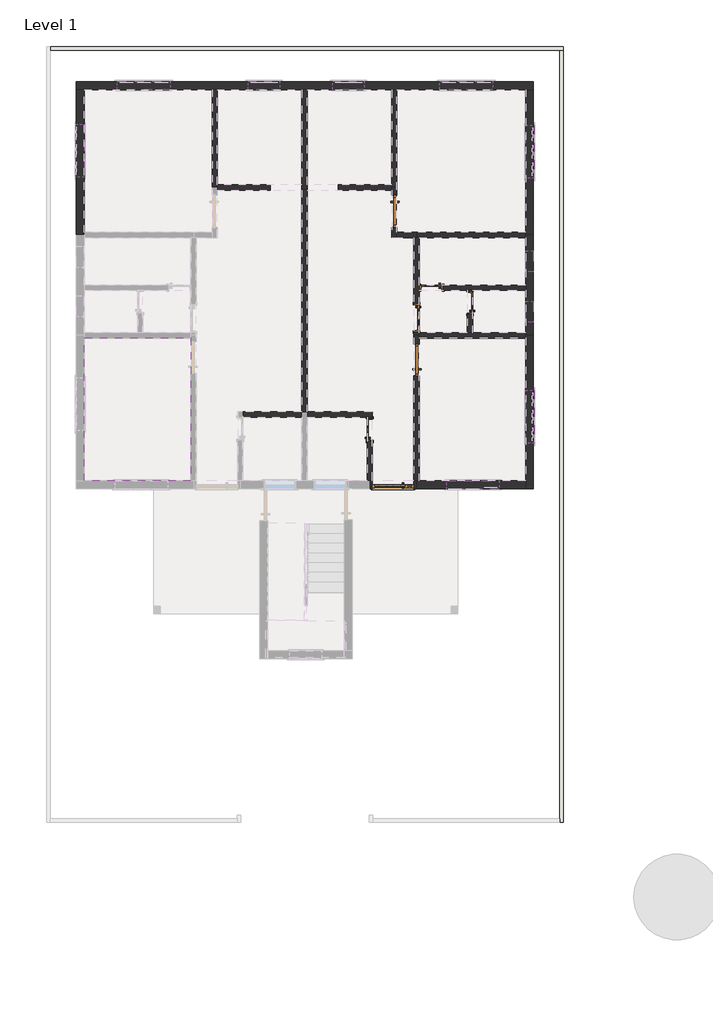
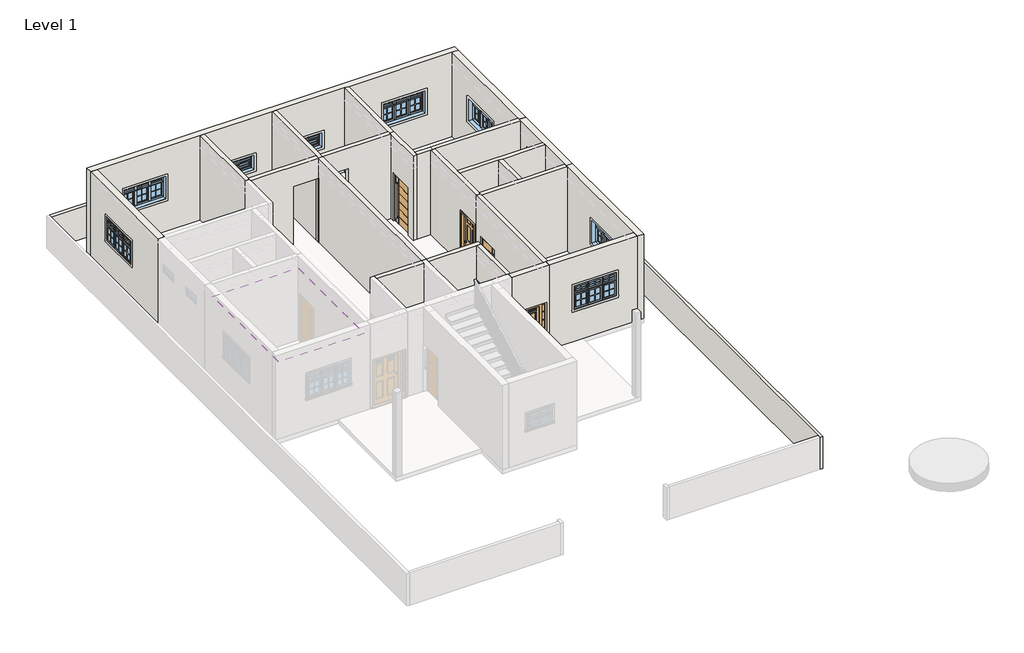
# One storey, part 2 of 4: 25 walls, 10 windows, 7 doors, 1 covering.
"""IFC4 building model written with IfcOpenShell, lengths in millimetres."""

from ifc_helpers import new_model, si_unit, frame, origin, place, context, project, spatial, polyline, outline, extrude, faceted_brep, transform, mapped, element, save
from components import door_3_ad1505b7, door_3_44036f4b, extsgl_w_side_panel_d749231e, m_door_interior_single_4_panel_wood_2_0346d007, m_door_interior_single_4_panel_wood_2_b7882c25, m_door_interior_single_6_panel_wood_750_x_2000mm_9b0189c3, fixed_2_8c8825d0, m_window_awning_double_vertical_3_7e34f04a, m_window_casement_triple_awning_triple_5_96d5a87e

model = new_model("IFC4")

# Units and contexts
model_context = context("Model", 3, world=origin())
ifc_project = project(units=[si_unit("LENGTHUNIT", "METRE", prefix="MILLI")], contexts=[model_context])

# Site, building, storey
site = spatial("IfcSite", under=ifc_project)
building = spatial("IfcBuilding", under=site)
storey = spatial("IfcBuildingStorey", under=building, Name="Level 1", Elevation=0.0)

# Covering
placement = place(None, origin())
element("IfcCovering", 1, ObjectType="2' x 4' ACT System", at=placement, inside=storey, context=model_context, shape_type="SweptSolid", body=[
    extrude(outline(polyline([(-10240.2299582, 8140.036641), (-13313.6299582, 8140.036641), (-13313.6299582, 12254.836641), (-10240.2299582, 12254.836641), (-10240.2299582, 8140.036641)])), frame((0.0, 0.0, 2743.2), z_axis=(0.0, 0.0, 1.0), x_axis=(1.0, 0.0, 0.0)), (0.0, 0.0, 1.0), 57.15),
])

# Doors
door_3_shape = door_3_ad1505b7(model_context)
element("IfcDoor", 2, ObjectType="3'", at=placement, inside=storey, context=model_context, shape_type="MappedRepresentation", body=[
    mapped(door_3_shape, transform((-4372.8299582, 15912.436641, 0.0), x_axis=(0.0, -1.0, 0.0), y_axis=(1.0, 0.0, 0.0), z_axis=(0.0, 0.0, 1.0))),
])
door_3_2_shape = door_3_44036f4b(model_context)
element("IfcDoor", 3, ObjectType="3'", at=placement, inside=storey, context=model_context, shape_type="MappedRepresentation", body=[
    mapped(door_3_2_shape, transform((-3737.8299582, 11619.836641, 0.0), x_axis=(0.0, 1.0, 0.0), y_axis=(-1.0, 0.0, 0.0), z_axis=(0.0, 0.0, 1.0))),
])
extsgl_w_side_panel_shape = extsgl_w_side_panel_d749231e(model_context)
element("IfcDoor", 4, ObjectType="ExtSgl w Side Panel", at=placement, inside=storey, context=model_context, shape_type="MappedRepresentation", body=[
    mapped(extsgl_w_side_panel_shape, transform((-4643.0299582, 8025.736641, 0.0), x_axis=(-1.0, 0.0, 0.0), y_axis=(0.0, -1.0, 0.0), z_axis=(0.0, 0.0, 1.0))),
])
m_door_interior_single_4_panel_wood_2_shape = m_door_interior_single_4_panel_wood_2_0346d007(model_context)
element("IfcDoor", 5, ObjectType="M_Door-Interior-Single-4_Panel-Wood : 2'", at=placement, inside=storey, context=model_context, shape_type="MappedRepresentation", body=[
    mapped(m_door_interior_single_4_panel_wood_2_shape, transform((-5087.2049582, 9613.236641, 0.0), x_axis=(0.0, 1.0, 0.0), y_axis=(-1.0, 0.0, 0.0), z_axis=(0.0, 0.0, 1.0))),
])
m_door_interior_single_4_panel_wood_2_2_shape = m_door_interior_single_4_panel_wood_2_b7882c25(model_context)
element("IfcDoor", 6, ObjectType="M_Door-Interior-Single-4_Panel-Wood : 2'", at=placement, inside=storey, context=model_context, shape_type="MappedRepresentation", body=[
    mapped(m_door_interior_single_4_panel_wood_2_2_shape, transform((-2185.2549582, 13270.836641, 0.0), x_axis=(0.0, 1.0, 0.0), y_axis=(-1.0, 0.0, 0.0), z_axis=(0.0, 0.0, 1.0))),
])
element("IfcDoor", 7, ObjectType="M_Door-Interior-Single-4_Panel-Wood : 2'", at=placement, inside=storey, context=model_context, shape_type="MappedRepresentation", body=[
    mapped(m_door_interior_single_4_panel_wood_2_2_shape, transform((-3306.0299582, 13705.811641, 0.0), x_axis=(-1.0, 0.0, 0.0), y_axis=(0.0, -1.0, 0.0), z_axis=(0.0, 0.0, 1.0))),
])
m_door_interior_single_6_panel_wood_750_x_2000mm_shape = m_door_interior_single_6_panel_wood_750_x_2000mm_9b0189c3(model_context)
element("IfcDoor", 8, ObjectType="M_Door-Interior-Single-6_Panel-Wood : 750 x 2000mm", at=placement, inside=storey, context=model_context, shape_type="MappedRepresentation", body=[
    mapped(m_door_interior_single_6_panel_wood_750_x_2000mm_shape, transform((-3734.6549582, 12839.036641, 0.0), x_axis=(0.0, -1.0, 0.0), y_axis=(1.0, 0.0, 0.0), z_axis=(0.0, 0.0, 1.0))),
])

# Walls
element("IfcWall", 9, ObjectType="Generic - 4\"", at=placement, inside=storey, context=model_context, shape_type="Brep", body=[
    faceted_brep([(-14304.2299582, 20560.636641, -152.4), (402.3700418, 20560.636641, -152.4), (503.9700418, 20560.636641, -152.4), (503.9700418, 20560.636641, 1066.8), (402.3700418, 20560.636641, 1066.8), (-14304.2299582, 20560.636641, 1066.8), (-14304.2299582, 20662.236641, -152.4), (-14304.2299582, 20662.236641, 1066.8), (503.9700418, 20662.236641, 1066.8), (503.9700418, 20662.236641, -152.4)], [[[0, 1, 2, 3, 4, 5]], [[6, 7, 8, 9]], [[2, 1, 0, 6, 9]], [[5, 4, 3, 8, 7]], [[0, 5, 7, 6]], [[3, 2, 9, 8]]]),
])
element("IfcWall", 10, ObjectType="Generic - 4\"", at=placement, inside=storey, context=model_context, shape_type="Brep", body=[
    faceted_brep([(402.3700418, 20560.636641, -152.4), (402.3700418, -1613.563359, -152.4), (402.3700418, -1715.163359, -152.4), (402.3700418, -1715.163359, 1066.8), (402.3700418, -1613.563359, 1066.8), (402.3700418, 20560.636641, 1066.8), (503.9700418, 20560.636641, -152.4), (503.9700418, 20560.636641, 1066.8), (503.9700418, -1715.163359, 1066.8), (503.9700418, -1715.163359, -152.4)], [[[0, 1, 2, 3, 4, 5]], [[6, 7, 8, 9]], [[2, 1, 0, 6, 9]], [[5, 4, 3, 8, 7]], [[0, 5, 7, 6]], [[3, 2, 9, 8]]]),
])
element("IfcWall", 11, ObjectType="Generic - 6\"", at=placement, inside=storey, context=model_context, shape_type="Brep", body=[
    faceted_brep([(-9630.6299582, 19417.636641, 0.0), (-9630.6299582, 16598.236641, 0.0), (-9630.6299582, 16598.236641, 3200.4), (-9630.6299582, 19417.636641, 3200.4), (-9478.2299582, 19417.636641, 0.0), (-9478.2299582, 19417.636641, 3200.4), (-9478.2299582, 16674.436641, 3200.4), (-9478.2299582, 16598.236641, 3200.4), (-9478.2299582, 16598.236641, 0.0), (-9478.2299582, 16674.436641, 0.0)], [[[0, 1, 2, 3]], [[4, 5, 6, 7, 8, 9]], [[1, 0, 4, 9, 8]], [[2, 1, 8, 7]], [[3, 2, 7, 6, 5]], [[0, 3, 5, 4]]]),
])
element("IfcWall", 12, ObjectType="Generic - 6\"", at=placement, inside=storey, context=model_context, shape_type="Brep", body=[
    faceted_brep([(-7039.8299582, 16522.036641, 0.0), (-7039.8299582, 16522.036641, 3200.4), (-9478.2299582, 16522.036641, 3200.4), (-9478.2299582, 16522.036641, 0.0), (-7956.9693204, 16522.036641, 0.0), (-7956.9693204, 16522.036641, 2438.4), (-7041.2238046, 16522.036641, 2438.4), (-7041.2238046, 16522.036641, 0.0), (-7039.8299582, 16674.436641, 3200.4), (-7039.8299582, 16674.436641, 0.0), (-7041.2238046, 16674.436641, 0.0), (-7041.2238046, 16674.436641, 2438.4), (-7956.9693204, 16674.436641, 2438.4), (-7956.9693204, 16674.436641, 0.0), (-9478.2299582, 16674.436641, 0.0), (-9478.2299582, 16674.436641, 3200.4), (-9478.2299582, 16598.236641, 0.0), (-7039.8299582, 16534.736641, 0.0), (-7039.8299582, 16534.736641, 3200.4), (-9478.2299582, 16598.236641, 3200.4)], [[[0, 1, 2, 3, 4, 5, 6, 7]], [[8, 9, 10, 11, 12, 13, 14, 15]], [[3, 16, 14, 13, 4]], [[9, 17, 0, 7, 10]], [[2, 1, 18, 8, 15, 19]], [[3, 2, 19, 15, 14, 16]], [[1, 0, 17, 9, 8, 18]], [[5, 12, 11, 6]], [[12, 5, 4, 13]], [[6, 11, 10, 7]]]),
])
element("IfcWall", 13, ObjectType="Generic - 6\"", at=placement, inside=storey, context=model_context, shape_type="Brep", body=[
    faceted_brep([(-7039.8299582, 19417.636641, 0.0), (-7039.8299582, 16674.436641, 0.0), (-7039.8299582, 16534.736641, 0.0), (-7039.8299582, 16534.736641, 3200.4), (-7039.8299582, 16674.436641, 3200.4), (-7039.8299582, 19417.636641, 3200.4), (-6887.4299582, 19417.636641, 0.0), (-6887.4299582, 19417.636641, 3200.4), (-6887.4299582, 16674.436641, 3200.4), (-6887.4299582, 16534.736641, 3200.4), (-6887.4299582, 16534.736641, 0.0), (-6887.4299582, 16674.436641, 0.0)], [[[0, 1, 2, 3, 4, 5]], [[6, 7, 8, 9, 10, 11]], [[2, 1, 0, 6, 11, 10]], [[3, 2, 10, 9]], [[5, 4, 3, 9, 8, 7]], [[0, 5, 7, 6]]]),
])
element("IfcWall", 14, ObjectType="Generic - 6\"", at=placement, inside=storey, context=model_context, shape_type="Brep", body=[
    faceted_brep([(-4449.0299582, 19417.636641, 0.0), (-4449.0299582, 16674.436641, 0.0), (-4449.0299582, 16598.236641, 0.0), (-4449.0299582, 16598.236641, 3200.4), (-4449.0299582, 16674.436641, 3200.4), (-4449.0299582, 19417.636641, 3200.4), (-4296.6299582, 19417.636641, 0.0), (-4296.6299582, 19417.636641, 3200.4), (-4296.6299582, 16598.236641, 3200.4), (-4296.6299582, 16598.236641, 0.0)], [[[0, 1, 2, 3, 4, 5]], [[6, 7, 8, 9]], [[2, 1, 0, 6, 9]], [[3, 2, 9, 8]], [[5, 4, 3, 8, 7]], [[0, 5, 7, 6]]]),
])
element("IfcWall", 15, ObjectType="Generic - 6\"", at=placement, inside=storey, context=model_context, shape_type="Brep", body=[
    faceted_brep([(-6887.4299582, 16674.436641, 0.0), (-6887.4299582, 16674.436641, 3200.4), (-4449.0299582, 16674.436641, 3200.4), (-4449.0299582, 16674.436641, 0.0), (-5985.1509554, 16674.436641, 0.0), (-5985.1509554, 16674.436641, 2438.4), (-6886.6436227, 16674.436641, 2438.4), (-6886.6436227, 16674.436641, 0.0), (-6887.4299582, 16522.036641, 3200.4), (-6887.4299582, 16522.036641, 0.0), (-6886.6436227, 16522.036641, 0.0), (-6886.6436227, 16522.036641, 2438.4), (-5985.1509554, 16522.036641, 2438.4), (-5985.1509554, 16522.036641, 0.0), (-4449.0299582, 16522.036641, 0.0), (-4449.0299582, 16522.036641, 3200.4), (-6887.4299582, 16534.736641, 0.0), (-4449.0299582, 16598.236641, 0.0), (-6887.4299582, 16534.736641, 3200.4), (-4449.0299582, 16598.236641, 3200.4)], [[[0, 1, 2, 3, 4, 5, 6, 7]], [[8, 9, 10, 11, 12, 13, 14, 15]], [[9, 16, 0, 7, 10]], [[3, 17, 14, 13, 4]], [[2, 1, 18, 8, 15, 19]], [[1, 0, 16, 9, 8, 18]], [[3, 2, 19, 15, 14, 17]], [[5, 12, 11, 6]], [[12, 5, 4, 13]], [[6, 11, 10, 7]]]),
])
element("IfcWall", 16, ObjectType="Generic - 6\"", at=placement, inside=storey, context=model_context, shape_type="Brep", body=[
    faceted_brep([(-4296.6299582, 15150.436641, 0.0), (-3814.0299582, 15150.436641, 0.0), (-3737.8299582, 15150.436641, 0.0), (-3737.8299582, 15150.436641, 3200.4), (-3814.0299582, 15150.436641, 3200.4), (-4296.6299582, 15150.436641, 3200.4), (-4296.6299582, 15302.836641, 0.0), (-4296.6299582, 15302.836641, 3200.4), (-3737.8299582, 15302.836641, 3200.4), (-3737.8299582, 15302.836641, 0.0)], [[[0, 1, 2, 3, 4, 5]], [[6, 7, 8, 9]], [[2, 1, 0, 6, 9]], [[3, 2, 9, 8]], [[5, 4, 3, 8, 7]], [[0, 5, 7, 6]]]),
])
element("IfcWall", 17, ObjectType="Generic - 6\"", at=placement, inside=storey, context=model_context, shape_type="Brep", body=[
    faceted_brep([(-3814.0299582, 12331.036641, 0.0), (-3814.0299582, 12331.036641, 3200.4), (-3814.0299582, 15150.436641, 3200.4), (-3814.0299582, 15150.436641, 0.0), (-3814.0299582, 13239.036641, 0.0), (-3814.0299582, 13239.036641, 2025.0), (-3814.0299582, 12439.036641, 2025.0), (-3814.0299582, 12439.036641, 0.0), (-3661.6299582, 12331.036641, 3200.4), (-3661.6299582, 12331.036641, 0.0), (-3661.6299582, 12407.236641, 0.0), (-3661.6299582, 12439.036641, 0.0), (-3661.6299582, 12439.036641, 2025.0), (-3661.6299582, 13239.036641, 2025.0), (-3661.6299582, 13239.036641, 0.0), (-3661.6299582, 13626.436641, 0.0), (-3661.6299582, 13778.836641, 0.0), (-3661.6299582, 15150.436641, 0.0), (-3661.6299582, 15150.436641, 3200.4), (-3661.6299582, 13778.836641, 3200.4), (-3661.6299582, 13626.436641, 3200.4), (-3661.6299582, 12407.236641, 3200.4), (-3737.8299582, 15150.436641, 0.0), (-3737.8299582, 15150.436641, 3200.4)], [[[0, 1, 2, 3, 4, 5, 6, 7]], [[8, 9, 10, 11, 12, 13, 14, 15, 16, 17, 18, 19, 20, 21]], [[3, 22, 17, 16, 15, 14, 4]], [[9, 0, 7, 11, 10]], [[1, 0, 9, 8]], [[2, 1, 8, 21, 20, 19, 18, 23]], [[3, 2, 23, 18, 17, 22]], [[6, 12, 11, 7]], [[12, 6, 5, 13]], [[13, 5, 4, 14]]]),
])
element("IfcWall", 18, ObjectType="Generic - 6\"", at=placement, inside=storey, context=model_context, shape_type="Brep", body=[
    faceted_brep([(-3661.6299582, 12254.836641, 0.0), (-588.2299582, 12254.836641, 0.0), (-588.2299582, 12254.836641, 3200.4), (-3661.6299582, 12254.836641, 3200.4), (-3661.6299582, 12407.236641, 0.0), (-3661.6299582, 12407.236641, 3200.4), (-2264.6299582, 12407.236641, 3200.4), (-2112.2299582, 12407.236641, 3200.4), (-588.2299582, 12407.236641, 3200.4), (-588.2299582, 12407.236641, 0.0), (-2112.2299582, 12407.236641, 0.0), (-2264.6299582, 12407.236641, 0.0), (-3661.6299582, 12331.036641, 0.0), (-588.2299582, 12331.036641, 0.0), (-588.2299582, 12331.036641, 3200.4), (-3661.6299582, 12331.036641, 3200.4)], [[[0, 1, 2, 3]], [[4, 5, 6, 7, 8, 9, 10, 11]], [[1, 0, 12, 4, 11, 10, 9, 13]], [[3, 2, 14, 8, 7, 6, 5, 15]], [[2, 1, 13, 9, 8, 14]], [[0, 3, 15, 5, 4, 12]]]),
])
element("IfcWall", 19, ObjectType="Generic - 6\"", at=placement, inside=storey, context=model_context, shape_type="SweptSolid", body=[
    extrude(outline(polyline([(12407.236641, 3200.4), (13626.436641, 3200.4), (13626.436641, 0.0), (13600.636641, 0.0), (13600.636641, 1853.8), (12941.036641, 1853.8), (12941.036641, 0.0), (12407.236641, 0.0), (12407.236641, 3200.4)])), frame((-2264.6299582, 0.0, 0.0), z_axis=(1.0, 0.0, 0.0), x_axis=(0.0, 1.0, 0.0)), (0.0, 0.0, 1.0), 152.4),
])
element("IfcWall", 20, ObjectType="Generic - 6\"", at=placement, inside=storey, context=model_context, shape_type="Brep", body=[
    faceted_brep([(-3661.6299582, 13778.836641, 3200.4), (-588.2299582, 13778.836641, 3200.4), (-588.2299582, 13778.836641, 0.0), (-2976.2299582, 13778.836641, 0.0), (-2976.2299582, 13778.836641, 1853.8), (-3635.8299582, 13778.836641, 1853.8), (-3635.8299582, 13778.836641, 0.0), (-3661.6299582, 13778.836641, 0.0), (-588.2299582, 13626.436641, 3200.4), (-2112.2299582, 13626.436641, 3200.4), (-2264.6299582, 13626.436641, 3200.4), (-3661.6299582, 13626.436641, 3200.4), (-3661.6299582, 13626.436641, 0.0), (-3635.8299582, 13626.436641, 0.0), (-3635.8299582, 13626.436641, 1853.8), (-2976.2299582, 13626.436641, 1853.8), (-2976.2299582, 13626.436641, 0.0), (-2264.6299582, 13626.436641, 0.0), (-2112.2299582, 13626.436641, 0.0), (-588.2299582, 13626.436641, 0.0)], [[[0, 1, 2, 3, 4, 5, 6, 7]], [[8, 9, 10, 11, 12, 13, 14, 15, 16, 17, 18, 19]], [[2, 19, 18, 17, 16, 3]], [[12, 7, 6, 13]], [[1, 0, 11, 10, 9, 8]], [[2, 1, 8, 19]], [[0, 7, 12, 11]], [[5, 14, 13, 6]], [[14, 5, 4, 15]], [[15, 4, 3, 16]]]),
])
element("IfcWall", 21, ObjectType="Generic - 6\"", at=placement, inside=storey, context=model_context, shape_type="Brep", body=[
    faceted_brep([(-8741.6299582, 9968.836641, 3200.4), (-8741.6299582, 9968.836641, 0.0), (-7039.8299582, 9968.836641, 0.0), (-7039.8299582, 9968.836641, 3200.4), (-8741.6299582, 10121.236641, 0.0), (-8741.6299582, 10121.236641, 3200.4), (-7039.8299582, 10121.236641, 3200.4), (-7039.8299582, 10121.236641, 0.0), (-7039.8299582, 10108.536641, 0.0), (-7039.8299582, 10108.536641, 3200.4)], [[[0, 1, 2, 3]], [[4, 5, 6, 7]], [[1, 4, 7, 8, 2]], [[5, 0, 3, 9, 6]], [[1, 0, 5, 4]], [[7, 6, 9, 3, 2, 8]]]),
    faceted_brep([(-5007.8299582, 9968.836641, 0.0), (-5007.8299582, 9968.836641, 3200.4), (-5160.2299582, 9968.836641, 3200.4), (-6887.4299582, 9968.836641, 3200.4), (-6887.4299582, 9968.836641, 0.0), (-5160.2299582, 9968.836641, 0.0), (-5007.8299582, 10121.236641, 3200.4), (-5007.8299582, 10121.236641, 0.0), (-6887.4299582, 10121.236641, 0.0), (-6887.4299582, 10121.236641, 3200.4), (-6887.4299582, 10108.536641, 0.0), (-6887.4299582, 10108.536641, 3200.4)], [[[0, 1, 2, 3, 4, 5]], [[6, 7, 8, 9]], [[7, 0, 5, 4, 10, 8]], [[1, 6, 9, 11, 3, 2]], [[1, 0, 7, 6]], [[9, 8, 10, 4, 3, 11]]]),
])
element("IfcWall", 22, ObjectType="Generic - 6\"", at=placement, inside=storey, context=model_context, shape_type="Brep", body=[
    faceted_brep([(-5160.2299582, 8140.036641, 3200.4), (-5160.2299582, 9968.836641, 3200.4), (-5160.2299582, 9968.836641, 0.0), (-5160.2299582, 9943.036641, 0.0), (-5160.2299582, 9943.036641, 1853.8), (-5160.2299582, 9283.436641, 1853.8), (-5160.2299582, 9283.436641, 0.0), (-5160.2299582, 8140.036641, 0.0), (-5007.8299582, 9968.836641, 3200.4), (-5007.8299582, 8140.036641, 3200.4), (-5007.8299582, 8140.036641, 1828.8), (-5007.8299582, 8140.036641, 0.0), (-5007.8299582, 9283.436641, 0.0), (-5007.8299582, 9283.436641, 1853.8), (-5007.8299582, 9943.036641, 1853.8), (-5007.8299582, 9943.036641, 0.0), (-5007.8299582, 9968.836641, 0.0), (-5084.0299582, 8140.036641, 0.0), (-5084.0299582, 8140.036641, 3200.4)], [[[0, 1, 2, 3, 4, 5, 6, 7]], [[8, 9, 10, 11, 12, 13, 14, 15, 16]], [[2, 16, 15, 3]], [[11, 17, 7, 6, 12]], [[1, 0, 18, 9, 8]], [[2, 1, 8, 16]], [[0, 7, 17, 11, 10, 9, 18]], [[14, 4, 3, 15]], [[4, 14, 13, 5]], [[5, 13, 12, 6]]]),
])
element("IfcWall", 23, ObjectType="Generic - 6\"", at=placement, inside=storey, context=model_context, shape_type="Brep", body=[
    faceted_brep([(-3814.0299582, 8140.036641, 3200.4), (-3814.0299582, 12331.036641, 3200.4), (-3814.0299582, 12331.036641, 0.0), (-3814.0299582, 12077.036641, 0.0), (-3814.0299582, 12077.036641, 1828.8), (-3814.0299582, 11162.636641, 1828.8), (-3814.0299582, 11162.636641, 0.0), (-3814.0299582, 8140.036641, 0.0), (-3661.6299582, 12331.036641, 3200.4), (-3661.6299582, 12254.836641, 3200.4), (-3661.6299582, 8140.036641, 3200.4), (-3661.6299582, 8140.036641, 0.0), (-3661.6299582, 11162.636641, 0.0), (-3661.6299582, 11162.636641, 1828.8), (-3661.6299582, 12077.036641, 1828.8), (-3661.6299582, 12077.036641, 0.0), (-3661.6299582, 12254.836641, 0.0), (-3661.6299582, 12331.036641, 0.0), (-3737.8299582, 8140.036641, 0.0), (-3758.6299582, 11162.636641, 0.0), (-3758.6299582, 11147.636641, 0.0), (-3681.6299582, 11147.636641, 0.0), (-3681.6299582, 11162.636641, 0.0), (-3681.6299582, 12077.036641, 0.0), (-3681.6299582, 12092.036641, 0.0), (-3758.6299582, 12092.036641, 0.0), (-3758.6299582, 12077.036641, 0.0), (-3737.8299582, 8140.036641, 3200.4), (-3681.6299582, 11162.636641, 1828.8), (-3681.6299582, 12077.036641, 1828.8), (-3758.6299582, 12077.036641, 1828.8), (-3758.6299582, 11162.636641, 1828.8), (-3681.6299582, 11147.636641, 1843.8), (-3758.6299582, 11147.636641, 1843.8), (-3758.6299582, 12092.036641, 1843.8), (-3681.6299582, 12092.036641, 1843.8)], [[[0, 1, 2, 3, 4, 5, 6, 7]], [[8, 9, 10, 11, 12, 13, 14, 15, 16, 17]], [[11, 18, 7, 6, 19, 20, 21, 22, 12]], [[2, 17, 16, 15, 23, 24, 25, 26, 3]], [[1, 0, 27, 10, 9, 8]], [[2, 1, 8, 17]], [[0, 7, 18, 11, 10, 27]], [[13, 28, 29, 14]], [[4, 30, 31, 5]], [[30, 4, 3, 26]], [[14, 29, 23, 15]], [[5, 31, 19, 6]], [[28, 13, 12, 22]], [[32, 33, 34, 35]], [[35, 34, 25, 24]], [[31, 30, 26, 25, 34, 33, 20, 19]], [[33, 32, 21, 20]], [[29, 28, 22, 21, 32, 35, 24, 23]]]),
])
element("IfcWall", 24, ObjectType="Generic - 6\"", at=placement, inside=storey, context=model_context, shape_type="Brep", body=[
    faceted_brep([(-7039.8299582, 16534.736641, 0.0), (-7039.8299582, 10121.236641, 0.0), (-7039.8299582, 10108.536641, 0.0), (-7039.8299582, 10108.536641, 3200.4), (-7039.8299582, 10121.236641, 3200.4), (-7039.8299582, 16534.736641, 3200.4), (-6887.4299582, 16534.736641, 0.0), (-6887.4299582, 16534.736641, 3200.4), (-6887.4299582, 10121.236641, 3200.4), (-6887.4299582, 10108.536641, 3200.4), (-6887.4299582, 10108.536641, 0.0), (-6887.4299582, 10121.236641, 0.0)], [[[0, 1, 2, 3, 4, 5]], [[6, 7, 8, 9, 10, 11]], [[2, 1, 0, 6, 11, 10]], [[3, 2, 10, 9]], [[5, 4, 3, 9, 8, 7]], [[0, 5, 7, 6]]]),
])
element("IfcWall", 25, ObjectType="Generic - 6\"", at=placement, inside=storey, context=model_context, shape_type="Brep", body=[
    faceted_brep([(-4449.0299582, 15150.436641, 3200.4), (-4449.0299582, 16522.036641, 3200.4), (-4449.0299582, 16598.236641, 3200.4), (-4449.0299582, 16598.236641, 0.0), (-4449.0299582, 16522.036641, 0.0), (-4449.0299582, 16369.636641, 0.0), (-4449.0299582, 16369.636641, 1828.8), (-4449.0299582, 15455.236641, 1828.8), (-4449.0299582, 15455.236641, 0.0), (-4449.0299582, 15150.436641, 0.0), (-4296.6299582, 16598.236641, 3200.4), (-4296.6299582, 15302.836641, 3200.4), (-4296.6299582, 15150.436641, 3200.4), (-4296.6299582, 15150.436641, 0.0), (-4296.6299582, 15302.836641, 0.0), (-4296.6299582, 15455.236641, 0.0), (-4296.6299582, 15455.236641, 1828.8), (-4296.6299582, 16369.636641, 1828.8), (-4296.6299582, 16369.636641, 0.0), (-4296.6299582, 16598.236641, 0.0), (-4393.6299582, 15455.236641, 0.0), (-4393.6299582, 15440.236641, 0.0), (-4316.6299582, 15440.236641, 0.0), (-4316.6299582, 15455.236641, 0.0), (-4316.6299582, 16369.636641, 0.0), (-4316.6299582, 16384.636641, 0.0), (-4393.6299582, 16384.636641, 0.0), (-4393.6299582, 16369.636641, 0.0), (-4393.6299582, 16369.636641, 1828.8), (-4393.6299582, 15455.236641, 1828.8), (-4316.6299582, 15455.236641, 1828.8), (-4316.6299582, 16369.636641, 1828.8), (-4316.6299582, 16384.636641, 1843.8), (-4316.6299582, 15440.236641, 1843.8), (-4393.6299582, 15440.236641, 1843.8), (-4393.6299582, 16384.636641, 1843.8)], [[[0, 1, 2, 3, 4, 5, 6, 7, 8, 9]], [[10, 11, 12, 13, 14, 15, 16, 17, 18, 19]], [[13, 9, 8, 20, 21, 22, 23, 15, 14]], [[3, 19, 18, 24, 25, 26, 27, 5, 4]], [[2, 1, 0, 12, 11, 10]], [[3, 2, 10, 19]], [[0, 9, 13, 12]], [[6, 28, 29, 7]], [[16, 30, 31, 17]], [[7, 29, 20, 8]], [[30, 16, 15, 23]], [[28, 6, 5, 27]], [[17, 31, 24, 18]], [[32, 33, 34, 35]], [[34, 33, 22, 21]], [[29, 28, 27, 26, 35, 34, 21, 20]], [[32, 35, 26, 25]], [[31, 30, 23, 22, 33, 32, 25, 24]]]),
])
element("IfcWall", 26, ObjectType="Generic - 6\"", at=placement, inside=storey, context=model_context, shape_type="Brep", body=[
    faceted_brep([(-3737.8299582, 15150.436641, 0.0), (-3661.6299582, 15150.436641, 0.0), (-588.2299582, 15150.436641, 0.0), (-588.2299582, 15150.436641, 3200.4), (-3661.6299582, 15150.436641, 3200.4), (-3737.8299582, 15150.436641, 3200.4), (-3737.8299582, 15302.836641, 0.0), (-3737.8299582, 15302.836641, 3200.4), (-588.2299582, 15302.836641, 3200.4), (-588.2299582, 15302.836641, 0.0), (-588.2299582, 15226.636641, 0.0), (-588.2299582, 15226.636641, 3200.4)], [[[0, 1, 2, 3, 4, 5]], [[6, 7, 8, 9]], [[2, 1, 0, 6, 9, 10]], [[5, 4, 3, 11, 8, 7]], [[0, 5, 7, 6]], [[3, 2, 10, 9, 8, 11]]]),
])
element("IfcWall", 27, ObjectType="Generic - 9\"", at=placement, inside=storey, context=model_context, shape_type="Brep", body=[
    faceted_brep([(-13542.2299582, 19417.636641, 0.0), (-13313.6299582, 19417.636641, 0.0), (-9630.6299582, 19417.636641, 0.0), (-9478.2299582, 19417.636641, 0.0), (-7039.8299582, 19417.636641, 0.0), (-6887.4299582, 19417.636641, 0.0), (-4449.0299582, 19417.636641, 0.0), (-4296.6299582, 19417.636641, 0.0), (-588.2299582, 19417.636641, 0.0), (-359.6299582, 19417.636641, 0.0), (-359.6299582, 19417.636641, 3200.4), (-588.2299582, 19417.636641, 3200.4), (-4296.6299582, 19417.636641, 3200.4), (-4449.0299582, 19417.636641, 3200.4), (-6887.4299582, 19417.636641, 3200.4), (-7039.8299582, 19417.636641, 3200.4), (-9478.2299582, 19417.636641, 3200.4), (-9630.6299582, 19417.636641, 3200.4), (-13313.6299582, 19417.636641, 3200.4), (-13542.2299582, 19417.636641, 3200.4), (-10837.1299582, 19417.636641, 2119.2), (-10837.1299582, 19417.636641, 1219.2), (-12361.1299582, 19417.636641, 1219.2), (-12361.1299582, 19417.636641, 2119.2), (-1540.7299582, 19417.636641, 2119.2), (-1540.7299582, 19417.636641, 1219.2), (-3064.7299582, 19417.636641, 1219.2), (-3064.7299582, 19417.636641, 2119.2), (-7674.8299582, 19417.636641, 1819.2), (-7674.8299582, 19417.636641, 1219.2), (-8589.2299582, 19417.636641, 1219.2), (-8589.2299582, 19417.636641, 1819.2), (-5236.4299582, 19417.636641, 1819.2), (-5236.4299582, 19417.636641, 1219.2), (-6150.8299582, 19417.636641, 1219.2), (-6150.8299582, 19417.636641, 1819.2), (-13542.2299582, 19646.236641, 0.0), (-13542.2299582, 19646.236641, 3200.4), (-359.6299582, 19646.236641, 3200.4), (-359.6299582, 19646.236641, 0.0), (-10837.1299582, 19646.236641, 2119.2), (-12361.1299582, 19646.236641, 2119.2), (-12361.1299582, 19646.236641, 1219.2), (-10837.1299582, 19646.236641, 1219.2), (-1540.7299582, 19646.236641, 2119.2), (-3064.7299582, 19646.236641, 2119.2), (-3064.7299582, 19646.236641, 1219.2), (-1540.7299582, 19646.236641, 1219.2), (-7674.8299582, 19646.236641, 1819.2), (-8589.2299582, 19646.236641, 1819.2), (-8589.2299582, 19646.236641, 1219.2), (-7674.8299582, 19646.236641, 1219.2), (-5236.4299582, 19646.236641, 1819.2), (-6150.8299582, 19646.236641, 1819.2), (-6150.8299582, 19646.236641, 1219.2), (-5236.4299582, 19646.236641, 1219.2)], [[[0, 1, 2, 3, 4, 5, 6, 7, 8, 9, 10, 11, 12, 13, 14, 15, 16, 17, 18, 19], [20, 21, 22, 23], [24, 25, 26, 27], [28, 29, 30, 31], [32, 33, 34, 35]], [[36, 37, 38, 39], [40, 41, 42, 43], [44, 45, 46, 47], [48, 49, 50, 51], [52, 53, 54, 55]], [[9, 8, 7, 6, 5, 4, 3, 2, 1, 0, 36, 39]], [[19, 18, 17, 16, 15, 14, 13, 12, 11, 10, 38, 37]], [[10, 9, 39, 38]], [[0, 19, 37, 36]], [[21, 20, 40, 43]], [[22, 21, 43, 42]], [[23, 22, 42, 41]], [[20, 23, 41, 40]], [[25, 24, 44, 47]], [[26, 25, 47, 46]], [[27, 26, 46, 45]], [[24, 27, 45, 44]], [[29, 28, 48, 51]], [[30, 29, 51, 50]], [[31, 30, 50, 49]], [[28, 31, 49, 48]], [[33, 32, 52, 55]], [[34, 33, 55, 54]], [[35, 34, 54, 53]], [[32, 35, 53, 52]]]),
])
element("IfcWall", 28, ObjectType="Generic - 9\"", at=placement, inside=storey, context=model_context, shape_type="Brep", body=[
    faceted_brep([(-588.2299582, 19417.636641, 0.0), (-588.2299582, 15302.836641, 0.0), (-588.2299582, 15226.636641, 0.0), (-588.2299582, 15226.636641, 3200.4), (-588.2299582, 15302.836641, 3200.4), (-588.2299582, 19417.636641, 3200.4), (-588.2299582, 16864.936641, 2119.2), (-588.2299582, 16864.936641, 1219.2), (-588.2299582, 18388.936641, 1219.2), (-588.2299582, 18388.936641, 2119.2), (-359.6299582, 19417.636641, 0.0), (-359.6299582, 19417.636641, 3200.4), (-359.6299582, 15226.636641, 3200.4), (-359.6299582, 15226.636641, 0.0), (-359.6299582, 16864.936641, 2119.2), (-359.6299582, 18388.936641, 2119.2), (-359.6299582, 18388.936641, 1219.2), (-359.6299582, 16864.936641, 1219.2)], [[[0, 1, 2, 3, 4, 5], [6, 7, 8, 9]], [[10, 11, 12, 13], [14, 15, 16, 17]], [[2, 1, 0, 10, 13]], [[3, 2, 13, 12]], [[5, 4, 3, 12, 11]], [[0, 5, 11, 10]], [[7, 6, 14, 17]], [[8, 7, 17, 16]], [[9, 8, 16, 15]], [[6, 9, 15, 14]]]),
])
element("IfcWall", 29, ObjectType="Generic - 9\"", at=placement, inside=storey, context=model_context, shape_type="Brep", body=[
    faceted_brep([(-588.2299582, 8140.036641, 0.0), (-3661.6299582, 8140.036641, 0.0), (-3737.8299582, 8140.036641, 0.0), (-3737.8299582, 8140.036641, 3200.4), (-3661.6299582, 8140.036641, 3200.4), (-588.2299582, 8140.036641, 3200.4), (-2867.8799582, 8140.036641, 2119.2), (-2867.8799582, 8140.036641, 1219.2), (-1343.8799582, 8140.036641, 1219.2), (-1343.8799582, 8140.036641, 2119.2), (-588.2299582, 7911.436641, 0.0), (-588.2299582, 7911.436641, 3200.4), (-3737.8299582, 7911.436641, 3200.4), (-3737.8299582, 7911.436641, 0.0), (-2867.8799582, 7911.436641, 2119.2), (-1343.8799582, 7911.436641, 2119.2), (-1343.8799582, 7911.436641, 1219.2), (-2867.8799582, 7911.436641, 1219.2)], [[[0, 1, 2, 3, 4, 5], [6, 7, 8, 9]], [[10, 11, 12, 13], [14, 15, 16, 17]], [[2, 1, 0, 10, 13]], [[3, 2, 13, 12]], [[5, 4, 3, 12, 11]], [[0, 5, 11, 10]], [[7, 6, 14, 17]], [[8, 7, 17, 16]], [[9, 8, 16, 15]], [[6, 9, 15, 14]]]),
])
element("IfcWall", 30, ObjectType="Generic - 9\"", at=placement, inside=storey, context=model_context, shape_type="Brep", body=[
    faceted_brep([(-588.2299582, 15226.636641, 0.0), (-588.2299582, 15150.436641, 0.0), (-588.2299582, 13778.836641, 0.0), (-588.2299582, 13626.436641, 0.0), (-588.2299582, 12407.236641, 0.0), (-588.2299582, 12331.036641, 0.0), (-588.2299582, 12331.036641, 3200.4), (-588.2299582, 12407.236641, 3200.4), (-588.2299582, 13626.436641, 3200.4), (-588.2299582, 13778.836641, 3200.4), (-588.2299582, 15150.436641, 3200.4), (-588.2299582, 15226.636641, 3200.4), (-588.2299582, 14159.836641, 2438.4), (-588.2299582, 14159.836641, 2133.6), (-588.2299582, 14769.436641, 2133.6), (-588.2299582, 14769.436641, 2438.4), (-588.2299582, 12712.036641, 2438.4), (-588.2299582, 12712.036641, 2133.6), (-588.2299582, 13321.636641, 2133.6), (-588.2299582, 13321.636641, 2438.4), (-359.6299582, 15226.636641, 0.0), (-359.6299582, 15226.636641, 3200.4), (-359.6299582, 12331.036641, 3200.4), (-359.6299582, 12331.036641, 0.0), (-359.6299582, 14159.836641, 2438.4), (-359.6299582, 14769.436641, 2438.4), (-359.6299582, 14769.436641, 2133.6), (-359.6299582, 14159.836641, 2133.6), (-359.6299582, 12712.036641, 2438.4), (-359.6299582, 13321.636641, 2438.4), (-359.6299582, 13321.636641, 2133.6), (-359.6299582, 12712.036641, 2133.6)], [[[0, 1, 2, 3, 4, 5, 6, 7, 8, 9, 10, 11], [12, 13, 14, 15], [16, 17, 18, 19]], [[20, 21, 22, 23], [24, 25, 26, 27], [28, 29, 30, 31]], [[5, 4, 3, 2, 1, 0, 20, 23]], [[6, 5, 23, 22]], [[11, 10, 9, 8, 7, 6, 22, 21]], [[0, 11, 21, 20]], [[12, 15, 25, 24]], [[15, 14, 26, 25]], [[14, 13, 27, 26]], [[13, 12, 24, 27]], [[16, 19, 29, 28]], [[19, 18, 30, 29]], [[18, 17, 31, 30]], [[17, 16, 28, 31]]]),
])
element("IfcWall", 31, ObjectType="Generic - 9\"", at=placement, inside=storey, context=model_context, shape_type="Brep", body=[
    faceted_brep([(-588.2299582, 12331.036641, 0.0), (-588.2299582, 12254.836641, 0.0), (-588.2299582, 8140.036641, 0.0), (-588.2299582, 7911.436641, 0.0), (-588.2299582, 7911.436641, 3200.4), (-588.2299582, 8140.036641, 3200.4), (-588.2299582, 12254.836641, 3200.4), (-588.2299582, 12331.036641, 3200.4), (-588.2299582, 9219.536641, 2119.2), (-588.2299582, 9219.536641, 1219.2), (-588.2299582, 10743.536641, 1219.2), (-588.2299582, 10743.536641, 2119.2), (-359.6299582, 12331.036641, 0.0), (-359.6299582, 12331.036641, 3200.4), (-359.6299582, 7911.436641, 3200.4), (-359.6299582, 7911.436641, 0.0), (-359.6299582, 9219.536641, 2119.2), (-359.6299582, 10743.536641, 2119.2), (-359.6299582, 10743.536641, 1219.2), (-359.6299582, 9219.536641, 1219.2)], [[[0, 1, 2, 3, 4, 5, 6, 7], [8, 9, 10, 11]], [[12, 13, 14, 15], [16, 17, 18, 19]], [[3, 2, 1, 0, 12, 15]], [[7, 6, 5, 4, 14, 13]], [[0, 7, 13, 12]], [[4, 3, 15, 14]], [[8, 11, 17, 16]], [[11, 10, 18, 17]], [[10, 9, 19, 18]], [[9, 8, 16, 19]]]),
])
element("IfcWall", 32, ObjectType="Generic - 9\"", at=placement, inside=storey, context=model_context, shape_type="Brep", body=[
    faceted_brep([(-5007.8299582, 8140.036641, 1828.8), (-5007.8299582, 8140.036641, 0.0), (-5084.0299582, 8140.036641, 0.0), (-5084.0299582, 8140.036641, 3200.4), (-5007.8299582, 8140.036641, 3200.4), (-3814.0299582, 8140.036641, 3200.4), (-3737.8299582, 8140.036641, 3200.4), (-3737.8299582, 8140.036641, 0.0), (-3814.0299582, 8140.036641, 0.0), (-3814.0299582, 8140.036641, 1828.8), (-5084.0299582, 7911.436641, 0.0), (-5007.8299582, 7911.436641, 0.0), (-5007.8299582, 7911.436641, 1828.8), (-3814.0299582, 7911.436641, 1828.8), (-3814.0299582, 7911.436641, 0.0), (-3737.8299582, 7911.436641, 0.0), (-3737.8299582, 7911.436641, 3200.4), (-5084.0299582, 7911.436641, 3200.4)], [[[0, 1, 2, 3, 4, 5, 6, 7, 8, 9]], [[10, 11, 12, 13, 14, 15, 16, 17]], [[8, 7, 15, 14]], [[2, 1, 11, 10]], [[3, 2, 10, 17]], [[6, 5, 4, 3, 17, 16]], [[7, 6, 16, 15]], [[13, 12, 0, 9]], [[12, 11, 1, 0]], [[14, 13, 9, 8]]]),
])
element("IfcWall", 33, ObjectType="Generic - 9\"", at=placement, inside=storey, context=model_context, shape_type="Brep", body=[
    faceted_brep([(-13313.6299582, 15226.636641, 0.0), (-13313.6299582, 15302.836641, 0.0), (-13313.6299582, 19417.636641, 0.0), (-13313.6299582, 19417.636641, 3200.4), (-13313.6299582, 15302.836641, 3200.4), (-13313.6299582, 15226.636641, 3200.4), (-13313.6299582, 18414.336641, 2119.2), (-13313.6299582, 18414.336641, 1219.2), (-13313.6299582, 16890.336641, 1219.2), (-13313.6299582, 16890.336641, 2119.2), (-13542.2299582, 15226.636641, 0.0), (-13542.2299582, 15226.636641, 3200.4), (-13542.2299582, 19417.636641, 3200.4), (-13542.2299582, 19417.636641, 0.0), (-13542.2299582, 18414.336641, 2119.2), (-13542.2299582, 16890.336641, 2119.2), (-13542.2299582, 16890.336641, 1219.2), (-13542.2299582, 18414.336641, 1219.2)], [[[0, 1, 2, 3, 4, 5], [6, 7, 8, 9]], [[10, 11, 12, 13], [14, 15, 16, 17]], [[2, 1, 0, 10, 13]], [[5, 4, 3, 12, 11]], [[0, 5, 11, 10]], [[3, 2, 13, 12]], [[6, 9, 15, 14]], [[9, 8, 16, 15]], [[8, 7, 17, 16]], [[7, 6, 14, 17]]]),
])

# Windows
fixed_2_shape = fixed_2_8c8825d0(model_context)
element("IfcWindow", 34, ObjectType="Fixed : 2'", at=placement, inside=storey, context=model_context, shape_type="MappedRepresentation", body=[
    mapped(fixed_2_shape, transform((-473.9299582, 14426.536641, 1219.2), x_axis=(0.0, -1.0, 0.0), y_axis=(1.0, 0.0, 0.0), z_axis=(0.0, 0.0, 1.0))),
])
element("IfcWindow", 35, ObjectType="Fixed : 2'", at=placement, inside=storey, context=model_context, shape_type="MappedRepresentation", body=[
    mapped(fixed_2_shape, transform((-473.9299582, 12978.736641, 1219.2), x_axis=(0.0, -1.0, 0.0), y_axis=(1.0, 0.0, 0.0), z_axis=(0.0, 0.0, 1.0))),
])
m_window_awning_double_vertical_3_shape = m_window_awning_double_vertical_3_7e34f04a(model_context)
element("IfcWindow", 36, ObjectType="M_Window-Awning-Double-Vertical : 4'", at=placement, inside=storey, context=model_context, shape_type="MappedRepresentation", body=[
    mapped(m_window_awning_double_vertical_3_shape, transform((-8132.0299582, 19531.936641, 319.2), x_axis=(1.0, 0.0, 0.0), y_axis=(0.0, 1.0, 0.0), z_axis=(0.0, 0.0, 1.0))),
])
element("IfcWindow", 37, ObjectType="M_Window-Awning-Double-Vertical : 4'", at=placement, inside=storey, context=model_context, shape_type="MappedRepresentation", body=[
    mapped(m_window_awning_double_vertical_3_shape, transform((-5693.6299582, 19531.936641, 319.2), x_axis=(1.0, 0.0, 0.0), y_axis=(0.0, 1.0, 0.0), z_axis=(0.0, 0.0, 1.0))),
])
m_window_casement_triple_awning_triple_5_shape = m_window_casement_triple_awning_triple_5_96d5a87e(model_context)
element("IfcWindow", 38, ObjectType="M_Window-Casement-Triple-Awning-Triple : 5'", at=placement, inside=storey, context=model_context, shape_type="MappedRepresentation", body=[
    mapped(m_window_casement_triple_awning_triple_5_shape, transform((-11599.1299582, 19531.936641, 319.2), x_axis=(1.0, 0.0, 0.0), y_axis=(0.0, 1.0, 0.0), z_axis=(0.0, 0.0, 1.0))),
])
element("IfcWindow", 39, ObjectType="M_Window-Casement-Triple-Awning-Triple : 5'", at=placement, inside=storey, context=model_context, shape_type="MappedRepresentation", body=[
    mapped(m_window_casement_triple_awning_triple_5_shape, transform((-13427.9299582, 17652.336641, 319.2), x_axis=(0.0, 1.0, 0.0), y_axis=(-1.0, 0.0, 0.0), z_axis=(0.0, 0.0, 1.0))),
])
element("IfcWindow", 40, ObjectType="M_Window-Casement-Triple-Awning-Triple : 5'", at=placement, inside=storey, context=model_context, shape_type="MappedRepresentation", body=[
    mapped(m_window_casement_triple_awning_triple_5_shape, transform((-2302.7299582, 19531.936641, 319.2), x_axis=(1.0, 0.0, 0.0), y_axis=(0.0, 1.0, 0.0), z_axis=(0.0, 0.0, 1.0))),
])
element("IfcWindow", 41, ObjectType="M_Window-Casement-Triple-Awning-Triple : 5'", at=placement, inside=storey, context=model_context, shape_type="MappedRepresentation", body=[
    mapped(m_window_casement_triple_awning_triple_5_shape, transform((-473.9299582, 17626.936641, 319.2), x_axis=(0.0, -1.0, 0.0), y_axis=(1.0, 0.0, 0.0), z_axis=(0.0, 0.0, 1.0))),
])
element("IfcWindow", 42, ObjectType="M_Window-Casement-Triple-Awning-Triple : 5'", at=placement, inside=storey, context=model_context, shape_type="MappedRepresentation", body=[
    mapped(m_window_casement_triple_awning_triple_5_shape, transform((-473.9299582, 9981.536641, 319.2), x_axis=(0.0, -1.0, 0.0), y_axis=(1.0, 0.0, 0.0), z_axis=(0.0, 0.0, 1.0))),
])
element("IfcWindow", 43, ObjectType="M_Window-Casement-Triple-Awning-Triple : 5'", at=placement, inside=storey, context=model_context, shape_type="MappedRepresentation", body=[
    mapped(m_window_casement_triple_awning_triple_5_shape, transform((-2105.8799582, 8025.736641, 319.2), x_axis=(-1.0, 0.0, 0.0), y_axis=(0.0, -1.0, 0.0), z_axis=(0.0, 0.0, 1.0))),
])

save(model, "model.ifc")

# Revit data of these elements
# Type "2' x 4' ACT System"
#   Assembly Code = "C3030210"
#   built-in parameter 1002203 = 1 (stored number, unit not read)
#   built-in parameter 1002202 = 1 (stored number, unit not read)
#   Layers, outside or top first: 0' - 1 5/8" "Default" (function 1); 0' - 0 5/8" "Acoustic Ceiling Tile 24 x 48" (function 5)
# Type "3'"
#   Type Mark = "9"
#   Water resistance = "up to Class E900, EN 12208:2001"
#   Uniclass2015Version = "v1.21"
#   Uniclass2015Reference = "Ss_25_30_20_30"
#   Uniclass2015Description = "Frame and door leaf system"
#   URL = "www.aluprof.com"
#   Type IFC Predefined Type = "USERDEFINED"
#   Right-hand / Left-hand door [instance default] = ""
#   Resistance to wind load = "up to Class C5/B5, EN 12210:2001"
#   Insert type = "ST"
#   Hardware [instance default] = ""
#   Product page = "https://aluprof.com/en/architects/offer/window-and-door-systems/panel-doors#visualisation"
#   Operation = "SinglePanelOutwardOpening"
#   Opening type = "Outward"
#   NBSReference = "25-50-20/125"
#   NBSDescription = "Frame and door leaf system"
#   Important = "The actual acceptable construction dimensions are dependent on the selection of profiles and hardware, glazing type, construction weight and the construction’s operating conditions. These should be determined by a suitably qualified person, and using ALUPROF’s calculation software"
#   IfcExportType = "USERDEFINED"
#   IfcExportAs = "IfcDoorType"
#   Handle type [instance default] = ""
#   Manufacturer = "ALUPROF SA"
#   Export Type to IFC As = "IfcDoorType"
#   Door sill type [instance default] = ""
#   Description = "External single-leaf panel door outward opening"
#   Model = "MB-86 ST Panel Door AD07"
#   Content of the recyclate in the material = "69.2%"
#   COBie.Type.WarrantyDurationParts = ""
#   COBie.Type.Name = ""
#   COBie.Type.Manufacturer = "ALUPROF SA"
#   COBie.Space.Name = ""
#   COBie.Floor.Name = ""
#   COBie.Facility.Name = ""
#   COBie.CreatedOn = ""
#   COBie.Component.WarrantyStartDate = ""
#   COBie.Component.Name = "MB-86 ST Panel Door AD07"
#   Burglar resistance = "RC2"
#   Air permeability = "up to Class 4, EN 12207:2001"
#   Width of the active leaf = 2' - 8.17717"
#   Placement in wall = 0' - 0.7874"
#   Thickness = 0' - 3.0315"
#   Height of the opening sash = 5' - 9.44094"
#   Handle Offset = 3' - 5.33858"
#   Rough Height = 6' - 2.40945"
#   Rough Width = 3' - 1.1811"
#   Height = 6' - 0"
#   Width = 3' - 0"
#   Construction depth = 0' - 3.0315"
#   Clear opening width = 2' - 3.94882"
#   Clear opening height = 5' - 8.47638"
#   Height of the array = 0' - 11.08136"
#   Schedule No. [instance default] = 1
#   Handrail [instance default] = yes
#   IsExternal = yes
#   Handle [instance default] = no
#   Door closer [instance default] = no
#   Function = 1
#   COBie.Type = yes
#   COBie = yes
#   Access control [instance default] = no
#   Panel = element 380416
#   Wall Closure = (empty or 0)
# Type "ExtSgl w Side Panel"
#   Type Mark = "14"
#   Operation = "SingleSwingRight"
#   Keynote = "L20"
#   Wrap Layers (Int) from Ext = 0' - 6.98819"
#   Wrap Layers (Ext) from Ext = 0' - 4.03543"
#   Thickness = 0' - 1.73228"
#   Stile Top of Lock rail = 3' - 3.37008"
#   Stile Top of Frieze Rail = 5' - 3.97638"
#   Stile Top Rail = 0' - 5.90551"
#   Stile Shutting = 0' - 4.92126"
#   Panelling Widths = 0' - 9.84252"
#   Stile Lock Rail = 0' - 6.88976"
#   Stile Intermediate/Frieze = 0' - 4.92126"
#   Stile Hanging = 0' - 4.92126"
#   Stile Bottom Rail = 0' - 6.88976"
#   Rough Width = 3' - 11"
#   Rough Height = 6' - 0"
#   O/A Frame Width = 0' - 2.51969"
#   Handle Z Distance = 3' - 3.37008"
#   Glazing Thickness = 0' - 0.94488"
#   Glazing Bar Thickness = 0' - 0.98425"
#   FrameWidth = 0' - 1.65354"
#   FrameOffset - External = 0' - 0.98425"
#   FrameDepth = 0' - 3.50394"
#   Door Panel Width = 2' - 11.70866"
#   Door Panel Thickness = 0' - 1.73228"
#   Door Panel Height = 5' - 7.66929"
#   Cill Thickness = 0' - 2.14567"
#   Cill Projection = 0' - 1.1811"
#   Handle X Distance = 0' - 2.95276"
#   Height = 6' - 0"
#   Structural Tolerance = 0' - 0.25591"
#   Tolerance = 0' - 0.11811"
#   Undercut = 0' - 0.15748"
#   Width = 3' - 11"
#   Cill Extension = 0' - 0.98425"
#   Cavity Closer Width = 0' - 1.9685"
#   Cavity Closer Offset from Ext = 0' - 4.03543"
#   Cavity Closer Depth = 0' - 3.34646"
#   Vis - SideLight Glazing Bars = yes
#   Vis - Ironmongery = yes
#   Vis - Cavity Closers = yes
#   Function = 1
#   Material Glass = Door - Glazing
#   Handle Style = element 390192
#   Material Door = Door - Panel
#   Material Ironmongery = Door - Handle
#   Wall Closure = (empty or 0)
# Type "M_Door-Interior-Single-4_Panel-Wood : 2'"
#   Type Mark = "13"
#   Assembly Code = "C1020300"
#   Analytic Construction = "Wooden"
#   Top Rail = 0' - 4.72441"
#   Thickness = 0' - 1.37795"
#   Thermal Resistance (R) = 2.5876 (h·ft²·°F)/BTU
#   Swing Angle [instance default] = 90.00°
#   Stiles = 0' - 4.72441"
#   Rough Width = 2' - 1.9685"
#   Rough Height = 6' - 0.98425"
#   Mullion = 0' - 4.52756"
#   Lock Rail = 0' - 7.87402"
#   Height = 6' - 0"
#   Width = 2' - 0"
#   Heat Transfer Coefficient (U) = 0.3865 BTU/(h·ft²·°F)
#   Bottom Rail = 0' - 9.05512"
#   Trim Material = Cherry
#   Panel Material = Cherry
#   Frame Material = Cherry
#   Door Handle Material = Aluminum
#   Visual Light Transmittance = 0
#   Solar Heat Gain Coefficient = 0
#   Wall Closure = (empty or 0)
#   Function = (empty or 0)
# Type "M_Door-Interior-Single-6_Panel-Wood : 750 x 2000mm"
#   Type Mark = "10"
#   Assembly Code = "C1020300"
#   Analytic Construction = "Wooden"
#   Top Rail = 0' - 4.72441"
#   Top Panel = 0' - 7.77559"
#   Thickness = 0' - 1.37795"
#   Thermal Resistance (R) = 2.5876 (h·ft²·°F)/BTU
#   Swing Angle [instance default] = 90.00°
#   Stiles = 0' - 4.72441"
#   Rough Width = 2' - 7.49606"
#   Rough Height = 6' - 7.72441"
#   Mullion = 0' - 4.52756"
#   Lock Rail = 0' - 7.87402"
#   Intermediate Rail = 0' - 4.52756"
#   Height = 6' - 6.74016"
#   Width = 2' - 5.52756"
#   Heat Transfer Coefficient (U) = 0.3865 BTU/(h·ft²·°F)
#   Bottom Rail = 0' - 9.05512"
#   Trim Material = Cherry
#   Panel Material = Cherry
#   Frame Material = Cherry
#   Door Handle Material = Aluminum
#   Visual Light Transmittance = 0
#   Solar Heat Gain Coefficient = 0
#   Wall Closure = (empty or 0)
#   Function = (empty or 0)
# Type "Generic - 4\""
#   Assembly Code = "B2010"
#   Layers, outside or top first: 0' - 4" no material (function 1)
# Type "Generic - 6\""
#   Assembly Code = "B2010"
#   Layers, outside or top first: 0' - 6" no material (function 1)
# Type "Generic - 9\""
#   Assembly Code = "B2010"
#   Layers, outside or top first: 0' - 9" no material (function 1)
# Type "Fixed : 2'"
#   Type Mark = "23"
#   Construction Type Id = "GSP4R"
#   Assembly Code = "B2020100"
#   Analytic Construction = "1/8 in Pilkington single glazing"
#   Visual Light Transmittance = 0.9
#   Solar Heat Gain Coefficient = 0.78
#   Heat Transfer Coefficient (U) = 0.6496 BTU/(h·ft²·°F)
#   Height = 1' - 0"
#   Default Sill Height = 3' - 0"
#   Width = 2' - 0"
#   Window Inset = 0' - 0 3/4"
#   Define Thermal Properties by = 1
#   Glass Pane Material = Glass
#   Sash Material = Sash
#   Wall Closure = (empty or 0)
# Type "M_Window-Awning-Double-Vertical : 4'"
#   Type Mark = "21"
#   Fire Rating = "0.5h"
#   Assembly Code = "B2020100"
#   Analytic Construction = "Double glazing - domestic"
#   Window Inset [instance default] = 0' - 0"
#   Wall Thickness [instance default] = 0' - 5.90551"
#   Visual Light Transmittance = 0.81
#   Top Sash Height Ratio = 0.5
#   Top Sash Height = 0' - 11.81102"
#   Thermal Resistance (R) = 1.8146 (h·ft²·°F)/BTU
#   Solar Heat Gain Coefficient = 0.76
#   Rough Width = 3' - 0.59055"
#   Rough Height = 2' - 0.2126"
#   Interior Wall Closure [instance default] = 0' - 2.15551"
#   Height = 1' - 11.62205"
#   Heat Transfer Coefficient (U) = 0.5511 BTU/(h·ft²·°F)
#   Frame Extension [instance default] = 0' - 0 1/4"
#   Exterior Wall Closure [instance default] = 0' - 1 1/4"
#   Extension Jamb [instance default] = 0' - 2.15551"
#   Default Sill Height = 2' - 11.43307"
#   Width = 3' - 0"
#   Top Muntin Visibility = yes
#   Interior Trim Visibility [instance default] = yes
#   Exterior Trim Visibility [instance default] = yes
#   Extension Jamb Visibility [instance default] = yes
#   Bottom Muntin Visibility = yes
#   Muntin Pattern = M_Muntin Pattern_2x2 : M_Muntin Pattern_2x2
#   Interior Trim Material = Wood - Stained
#   Interior Trim = M_Trim-Window-Interior-Flat : Picture Frame
#   Interior Frame Material = Wood - Stained
#   Glass Panel Material = Glass
#   Exterior Trim Material = Clad - White
#   Exterior Trim = M_Trim-Window-Exterior-Flat : with Sill
#   Exterior Frame Material = Clad - White
#   Wall Closure = (empty or 0)
# Type "M_Window-Casement-Triple-Awning-Triple : 5'"
#   Type Mark = "19"
#   Fire Rating = "0.5h"
#   Assembly Code = "B2020100"
#   Analytic Construction = "Double glazing - domestic"
#   Window Inset [instance default] = 0' - 0"
#   Wall Thickness [instance default] = 0' - 5.90551"
#   One Third Width = 1' - 8"
#   Visual Light Transmittance = 0.81
#   Transom Height = 0' - 11.81102"
#   Thermal Resistance (R) = 1.8146 (h·ft²·°F)/BTU
#   Solar Heat Gain Coefficient = 0.76
#   Sash Width = 1' - 7.16667"
#   Rough Width = 5' - 0.59055"
#   Rough Height = 3' - 0.02362"
#   Open Window Height = 1' - 11.62205"
#   Frame Extension [instance default] = 0' - 0 1/4"
#   Interior Wall Closure [instance default] = 0' - 2.15551"
#   Height = 2' - 11.43307"
#   Heat Transfer Coefficient (U) = 0.5511 BTU/(h·ft²·°F)
#   Exterior Wall Closure [instance default] = 0' - 1 1/4"
#   Extension Jamb [instance default] = 0' - 2.15551"
#   Default Sill Height = 2' - 11.43307"
#   Width = 5' - 0"
#   Top Side Muntin Visibility = yes
#   Top Middle Muntin Visibility = yes
#   Bottom Side Muntin Visibility = yes
#   Bottom Middle Muntin Visibility = yes
#   Interior Trim Visibility [instance default] = yes
#   Exterior Trim Visibility [instance default] = yes
#   Extension Jamb Visibility [instance default] = yes
#   Muntin Pattern = M_Muntin Pattern_2x2 : M_Muntin Pattern_2x2
#   Interior Trim Material = Wood - Stained
#   Interior Trim = M_Trim-Window-Interior-Flat : Picture Frame
#   Interior Frame Material = Wood - Stained
#   Glass Panel Material = Glass
#   Exterior Trim Material = Clad - White
#   Exterior Trim = M_Trim-Window-Exterior-Flat : with Sill
#   Exterior Frame Material = Clad - White
#   Wall Closure = (empty or 0)
# Element 1 (IfcCovering, "2' x 4' ACT System")
#   Height Offset From Level = 9' - 0"
#   Phase Created = New Construction
#   Materials on its faces: "Acoustic Ceiling Tile 24 x 48", "Default"
# Elements 2, 3 (IfcDoor, "3'")
#   Right-hand / Left-hand door = ""
#   Hardware = ""
#   Handle type = ""
#   Door sill type = ""
#   Schedule No. = 1
#   Handrail = yes
#   Handle = no
#   Door closer = no
#   Access control = no
#   Phase Created = New Construction
# Element 4 (IfcDoor, "ExtSgl w Side Panel")
#   Phase Created = New Construction
#   Materials on its faces: "Door - Panel", "Door - Handle", "Door - Glazing"
# Elements 5, 6, 7 (IfcDoor, "M_Door-Interior-Single-4_Panel-Wood : 2'")
#   Swing Angle = 90.00°
#   Phase Created = New Construction
#   Materials on its faces: "Cherry", "Aluminum"
# Element 8 (IfcDoor, "M_Door-Interior-Single-6_Panel-Wood : 750 x 2000mm")
#   Swing Angle = 90.00°
#   Phase Created = New Construction
#   Materials on its faces: "Cherry", "Aluminum"
# Elements 9, 10 (IfcWall, "Generic - 4\"")
#   built-in parameter 1001111 = -0' - 6"
#   Top Offset = 0' - 0"
#   Base Offset = -0' - 6"
#   Unconnected Height = 4' - 0"
#   wall height = 4' - 0"
#   Phase Created = New Construction
#   Base Constraint = Level 1
#   Materials on its faces: "LVW1", "Default Wall"
# Elements 11, 23 (IfcWall, "Generic - 6\"")
#   Top Offset = 0' - 0"
#   Base Offset = 0' - 0"
#   Unconnected Height = 10' - 6"
#   wall height = 10' - 6"
#   Phase Created = New Construction
#   Base Constraint = Level 1
#   Materials on its faces: "Default Wall", "BED ROOM WALL 1"
# Elements 12, 14, 16, 25 (IfcWall, "Generic - 6\"")
#   Top Offset = 0' - 0"
#   Base Offset = 0' - 0"
#   Unconnected Height = 10' - 6"
#   wall height = 10' - 6"
#   Phase Created = New Construction
#   Base Constraint = Level 1
#   Materials on its faces: "Default Wall", "BED ROOM WALL 2"
# Elements 13, 15 (IfcWall, "Generic - 6\"")
#   Top Offset = 0' - 0"
#   Base Offset = 0' - 0"
#   Unconnected Height = 10' - 6"
#   wall height = 10' - 6"
#   Phase Created = New Construction
#   Base Constraint = Level 1
#   Materials on its faces: "Default Wall", "BED ROOM WALL 2", "BED ROOM WALL 1"
# Elements 17, 19, 20, 21, 22 (IfcWall, "Generic - 6\"")
#   Top Offset = 0' - 0"
#   Base Offset = 0' - 0"
#   Unconnected Height = 10' - 6"
#   wall height = 10' - 6"
#   Phase Created = New Construction
#   Base Constraint = Level 1
#   Materials on its faces: "Default Wall", "BAW1"
# Element 18 (IfcWall, "Generic - 6\"")
#   Top Offset = 0' - 0"
#   Base Offset = 0' - 0"
#   Unconnected Height = 10' - 6"
#   wall height = 10' - 6"
#   Phase Created = New Construction
#   Base Constraint = Level 1
#   Materials on its faces: "Default Wall", "BED ROOM WALL 2", "BAW1"
# Element 24 (IfcWall, "Generic - 6\"")
#   Top Offset = 0' - 0"
#   Base Offset = 0' - 0"
#   Unconnected Height = 10' - 6"
#   wall height = 10' - 6"
#   Phase Created = New Construction
#   Base Constraint = Level 1
#   Materials on its faces: "Default Wall"
# Element 26 (IfcWall, "Generic - 6\"")
#   Top Offset = 0' - 0"
#   Base Offset = 0' - 0"
#   Unconnected Height = 10' - 6"
#   wall height = 10' - 6"
#   Phase Created = New Construction
#   Base Constraint = Level 1
#   Materials on its faces: "Default Wall", "BAW1", "BED ROOM WALL 2"
# Element 27 (IfcWall, "Generic - 9\"")
#   Top Offset = 0' - 0"
#   Base Offset = 0' - 0"
#   Unconnected Height = 10' - 6"
#   wall height = 10' - 6"
#   Phase Created = New Construction
#   Base Constraint = Level 1
#   Materials on its faces: "Default Wall", "LVW1", "BED ROOM WALL 1"
# Element 28 (IfcWall, "Generic - 9\"")
#   Top Offset = 0' - 0"
#   Base Offset = 0' - 0"
#   Unconnected Height = 10' - 6"
#   wall height = 10' - 6"
#   Phase Created = New Construction
#   Base Constraint = Level 1
#   Materials on its faces: "Default Wall", "BED ROOM WALL 1", "LVW1"
# Element 29 (IfcWall, "Generic - 9\"")
#   Top Offset = 0' - 0"
#   Base Offset = 0' - 0"
#   Unconnected Height = 10' - 6"
#   wall height = 10' - 6"
#   Phase Created = New Construction
#   Base Constraint = Level 1
#   Materials on its faces: "Default Wall", "BED ROOM WALL 1"
# Element 30 (IfcWall, "Generic - 9\"")
#   Top Offset = 0' - 0"
#   Base Offset = 0' - 0"
#   Unconnected Height = 10' - 6"
#   wall height = 10' - 6"
#   Phase Created = New Construction
#   Base Constraint = Level 1
#   Materials on its faces: "Default Wall", "BAW2", "LVW1"
# Elements 31, 33 (IfcWall, "Generic - 9\"")
#   Top Offset = 0' - 0"
#   Base Offset = 0' - 0"
#   Unconnected Height = 10' - 6"
#   wall height = 10' - 6"
#   Phase Created = New Construction
#   Base Constraint = Level 1
#   Materials on its faces: "Default Wall", "BED ROOM WALL 2", "LVW1"
# Element 32 (IfcWall, "Generic - 9\"")
#   Top Offset = 0' - 0"
#   Base Offset = 0' - 0"
#   Unconnected Height = 10' - 6"
#   wall height = 10' - 6"
#   Phase Created = New Construction
#   Base Constraint = Level 1
#   Materials on its faces: "Default Wall"
# Element 34 (IfcWindow, "Fixed : 2'")
#   Mark = "15"
#   Phase Created = New Construction
#   Materials on its faces: "Sash", "Glass"
# Element 35 (IfcWindow, "Fixed : 2'")
#   Mark = "16"
#   Phase Created = New Construction
#   Materials on its faces: "Sash", "Glass"
# Element 36 (IfcWindow, "M_Window-Awning-Double-Vertical : 4'")
#   Mark = "9"
#   Window Inset = 0' - 0"
#   Interior Wall Closure = 0' - 2.15551"
#   Frame Extension = 0' - 0 1/4"
#   Exterior Wall Closure = 0' - 1 1/4"
#   Interior Trim Visibility = yes
#   Exterior Trim Visibility = yes
#   Phase Created = New Construction
#   Materials on its faces: "Wood - Stained", "Glass", "Clad - White"
# Element 37 (IfcWindow, "M_Window-Awning-Double-Vertical : 4'")
#   Mark = "10"
#   Window Inset = 0' - 0"
#   Interior Wall Closure = 0' - 2.15551"
#   Frame Extension = 0' - 0 1/4"
#   Exterior Wall Closure = 0' - 1 1/4"
#   Interior Trim Visibility = yes
#   Exterior Trim Visibility = yes
#   Phase Created = New Construction
#   Materials on its faces: "Wood - Stained", "Glass", "Clad - White"
# Element 38 (IfcWindow, "M_Window-Casement-Triple-Awning-Triple : 5'")
#   Mark = "1"
#   Window Inset = 0' - 0"
